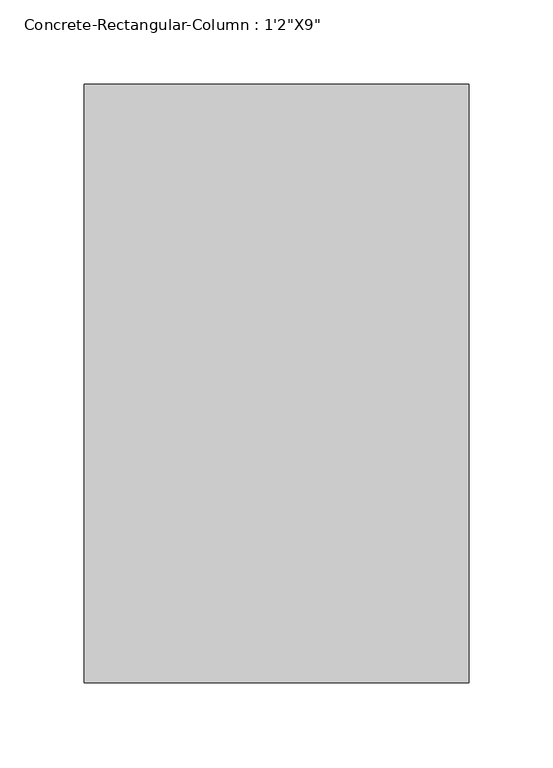
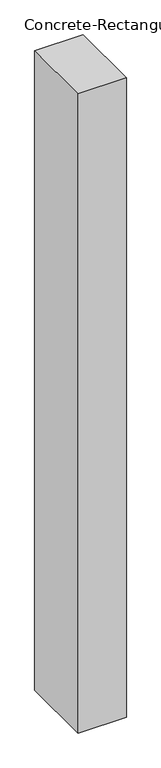
"""IFC4 building model written with IfcOpenShell, lengths in millimetres: column geometry."""

from ifc_helpers import new_model, si_unit, frame, origin, place, context, project, spatial, polyline, outline, extrude, source, transform, mapped, element, save


def column_4a663ebe(model_context):
    return source(origin(), model_context, "Body", "SweptSolid", [
        extrude(outline(polyline([(114.3, 177.8), (114.3, -177.8), (-114.3, -177.8), (-114.3, 177.8), (114.3, 177.8)])), frame((0.0, 0.0, 3200.4), z_axis=(0.0, 0.0, 1.0), x_axis=(1.0, 0.0, 0.0)), (0.0, 0.0, 1.0), 3200.4),
    ])


if __name__ == "__main__":
    model = new_model("IFC4")
    model_context = context("Model", 3, world=origin())
    ifc_project = project(units=[si_unit("LENGTHUNIT", "METRE", prefix="MILLI")], contexts=[model_context])
    site = spatial("IfcSite", under=ifc_project)
    building = spatial("IfcBuilding", under=site)
    placement = place(None, origin())
    column_shape = column_4a663ebe(model_context)
    element("IfcColumn", 1, ObjectType="Concrete-Rectangular-Column : 1'2\"X9\"", at=placement, inside=building, context=model_context, shape_type="MappedRepresentation", body=[
        mapped(column_shape, transform((0.0, 0.0, 0.0), x_axis=(1.0, 0.0, 0.0), y_axis=(0.0, 1.0, 0.0), z_axis=(0.0, 0.0, 1.0))),
    ])
    save(model, "model.ifc")

# Revit data of these elements
# Type "Concrete-Rectangular-Column : 1'2\"X9\""
#   Assembly Code = "B10"
#   b = 0' - 9"
#   h = 1' - 2"
#   Structural Material [instance default] = Concrete, Cast-in-Place gray
# Element 1 (IfcColumn, "Concrete-Rectangular-Column : 1'2\"X9\"")
#   Materials on its faces: "Concrete, Cast-in-Place gray"
# Materials
#   "Concrete, Cast-in-Place gray": class "Concrete", colour RGB 192 192 192, transparency 0, Description = "Cast-in-place concrete", Cost = 0
